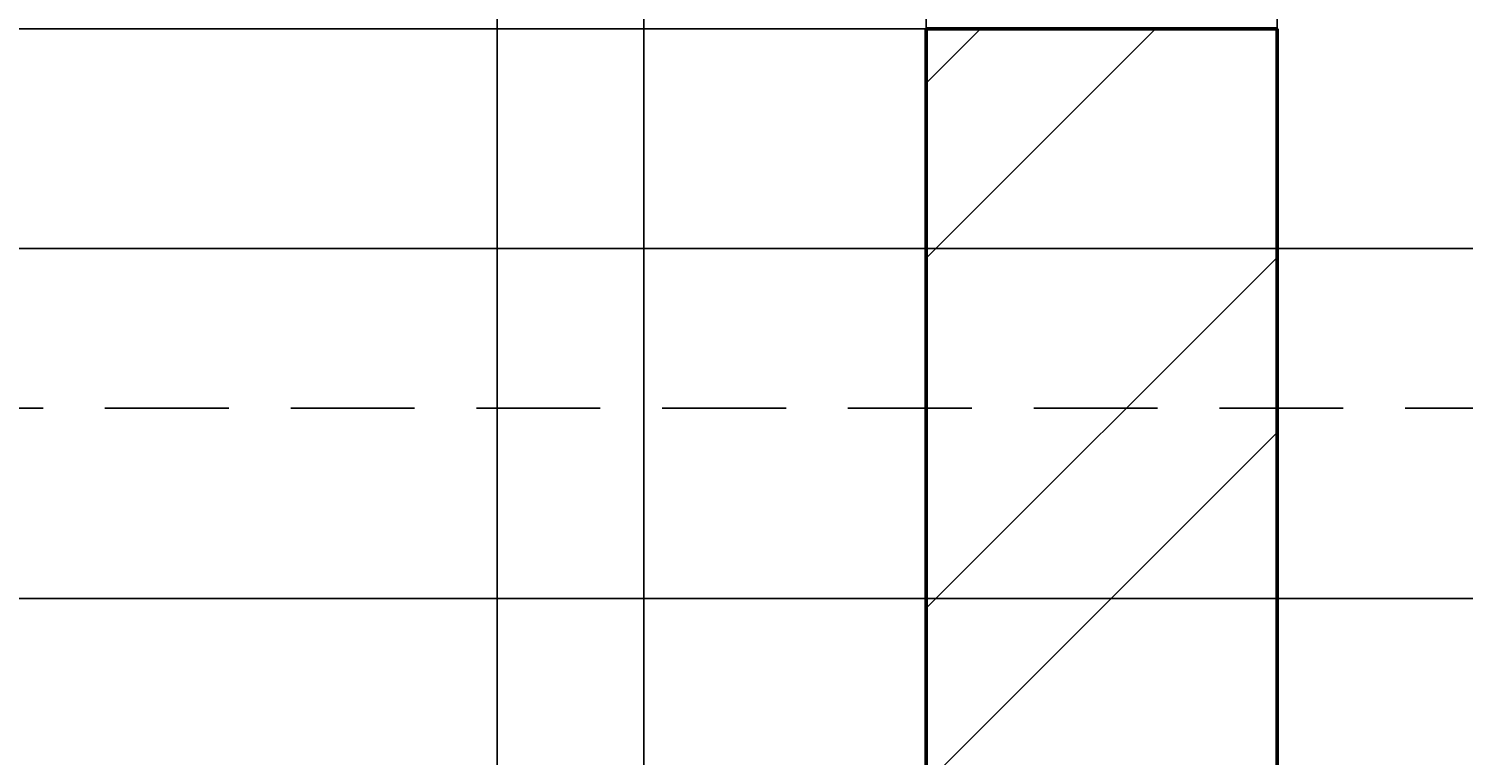
# Model space of a CAD drawing. Units: inches. Extents: x 2812 to 3051, y 1398 to 1659.
# Tile 22 of 65: x 2929 to 2966, y 1453 to 1472. Entities that reach past the tile are written whole.
import ezdxf

# ---------------------------------------------------------------- set-up
doc = ezdxf.new("R2010")
doc.units = ezdxf.units.IN
doc.linetypes.add('HIDDEN2', pattern=[4.7625, 3.175, -1.5875])
for name, color, linetype, lineweight in [('A-ANNO-DIMS', 2, 'Continuous', 18), ('S-CONC', 7, 'Continuous', 50), ('S-CONC-HIDN', 8, 'HIDDEN2', 25), ('S-CONC-PATT', 8, 'Continuous', 18)]:
    doc.layers.add(name, color=color, linetype=linetype, lineweight=lineweight)
doc.styles.get("Standard").update_dxf_attribs({"font": 'arial.ttf'})
doc.dimstyles.get("Standard").update_dxf_attribs({"dimtxt": 0.18, "dimasz": 0.18, "dimexe": 0.18, "dimexo": 0.0625, "dimgap": 0.09, "dimtad": 0, "dimtih": 1, "dimtoh": 1, "dimdec": 4, "dimzin": 0, "dimdsep": 46, "dimtxsty": 'Standard', "dimcen": 0.09, "dimadec": 0, "dimazin": 0, "dimtfac": 1, "dimtdec": 4, "dimtofl": 0, "dimtmove": 0, "dimatfit": 3, "dimfxl": 1, "dimtolj": 1, "dimtzin": 0, "dimarcsym": 0})

# ---------------------------------------------------------------- blocks, each defined once
blk = doc.blocks.new('*D30')
at = {"layer": 'A-ANNO-DIMS', "color": 0, "lineweight": -2, "transparency": 16777216}
for p, q in [((2945.147, 1598.692), (2945.147, 1397.505)), ((2952.385, 1559.757), (2952.385, 1397.505)), ((2945.327, 1397.685), (2948.373, 1397.685)), ((2952.205, 1397.685), (2949.159, 1397.685))]:
    blk.add_line(p, q, dxfattribs=at)
at = {"layer": 'A-ANNO-DIMS', "color": 0, "transparency": 16777216}
for points in [[(2945.327, 1397.715), (2945.327, 1397.655), (2945.147, 1397.685)], [(2952.205, 1397.715), (2952.205, 1397.655), (2952.385, 1397.685)]]:
    blk.add_solid(points, dxfattribs=at)
at = {"layer": 'Defpoints', "color": 0, "transparency": 16777216}
for p in [(2945.147, 1598.754), (2952.385, 1559.82), (2952.385, 1397.685)]:
    blk.add_point(p, dxfattribs=at)
at = {"layer": 'A-ANNO-DIMS', "color": 0, "transparency": 16777216, "insert": (2948.766, 1397.685), "char_height": 0.18, "attachment_point": 5}
blk.add_mtext('\\A1;7.238', dxfattribs=at)
blk = doc.blocks.new('*D31')
at = {"layer": 'A-ANNO-DIMS', "color": 0, "lineweight": -2, "transparency": 16777216}
for p, q in [((2972.272, 1594.192), (2972.272, 1397.505)), ((2961.385, 1559.757), (2961.385, 1397.505)), ((2961.565, 1397.685), (2966.373, 1397.685)), ((2972.092, 1397.685), (2967.283, 1397.685))]:
    blk.add_line(p, q, dxfattribs=at)
at = {"layer": 'A-ANNO-DIMS', "color": 0, "transparency": 16777216}
for points in [[(2961.565, 1397.715), (2961.565, 1397.655), (2961.385, 1397.685)], [(2972.092, 1397.715), (2972.092, 1397.655), (2972.272, 1397.685)]]:
    blk.add_solid(points, dxfattribs=at)
at = {"layer": 'Defpoints', "color": 0, "transparency": 16777216}
for p in [(2972.272, 1594.254), (2961.385, 1559.82), (2972.272, 1397.685)]:
    blk.add_point(p, dxfattribs=at)
at = {"layer": 'A-ANNO-DIMS', "color": 0, "transparency": 16777216, "insert": (2966.828, 1397.685), "char_height": 0.18, "attachment_point": 5}
blk.add_mtext('\\A1;10.887', dxfattribs=at)
blk = doc.blocks.new('*D45')
at = {"layer": 'A-ANNO-DIMS', "color": 0, "lineweight": -2, "transparency": 16777216}
for p, q in [((2896.385, 1487.973), (2896.385, 1397.505)), ((2941.385, 1487.973), (2941.385, 1397.505)), ((2896.565, 1397.685), (2918.662, 1397.685)), ((2941.205, 1397.685), (2919.108, 1397.685))]:
    blk.add_line(p, q, dxfattribs=at)
at = {"layer": 'A-ANNO-DIMS', "color": 0, "transparency": 16777216}
for points in [[(2896.565, 1397.715), (2896.565, 1397.655), (2896.385, 1397.685)], [(2941.205, 1397.715), (2941.205, 1397.655), (2941.385, 1397.685)]]:
    blk.add_solid(points, dxfattribs=at)
at = {"layer": 'Defpoints', "color": 0, "transparency": 16777216}
for p in [(2896.385, 1488.035), (2941.385, 1488.035), (2941.385, 1397.685)]:
    blk.add_point(p, dxfattribs=at)
at = {"layer": 'A-ANNO-DIMS', "color": 0, "transparency": 16777216, "insert": (2918.885, 1397.685), "char_height": 0.18, "attachment_point": 5}
blk.add_mtext('\\A1;45', dxfattribs=at)
blk = doc.blocks.new('*D46')
at = {"layer": 'A-ANNO-DIMS', "color": 0, "lineweight": -2, "transparency": 16777216}
for p, q in [((2941.385, 1487.973), (2941.385, 1397.505)), ((2970.385, 1487.973), (2970.385, 1397.505)), ((2941.565, 1397.685), (2955.664, 1397.685)), ((2970.205, 1397.685), (2956.106, 1397.685))]:
    blk.add_line(p, q, dxfattribs=at)
at = {"layer": 'A-ANNO-DIMS', "color": 0, "transparency": 16777216}
for points in [[(2941.565, 1397.715), (2941.565, 1397.655), (2941.385, 1397.685)], [(2970.205, 1397.715), (2970.205, 1397.655), (2970.385, 1397.685)]]:
    blk.add_solid(points, dxfattribs=at)
at = {"layer": 'Defpoints', "color": 0, "transparency": 16777216}
for p in [(2941.385, 1488.035), (2970.385, 1488.035), (2970.385, 1397.685)]:
    blk.add_point(p, dxfattribs=at)
at = {"layer": 'A-ANNO-DIMS', "color": 0, "transparency": 16777216, "insert": (2955.885, 1397.685), "char_height": 0.18, "attachment_point": 5}
blk.add_mtext('\\A1;29', dxfattribs=at)
blk = doc.blocks.new('*D67')
at = {"layer": 'A-ANNO-DIMS', "color": 0, "lineweight": -2, "transparency": 16777216}
for p, q in [((2906.065, 1457.426), (3051.178, 1457.426)), ((3050.998, 1457.246), (3050.998, 1452.608)), ((3050.998, 1447.606), (3050.998, 1452.245)), ((2914.018, 1447.426), (3051.178, 1447.426))]:
    blk.add_line(p, q, dxfattribs=at)
at = {"layer": 'A-ANNO-DIMS', "color": 0, "transparency": 16777216}
for points in [[(3050.968, 1457.246), (3051.028, 1457.246), (3050.998, 1457.426)], [(3050.968, 1447.606), (3051.028, 1447.606), (3050.998, 1447.426)]]:
    blk.add_solid(points, dxfattribs=at)
at = {"layer": 'Defpoints', "color": 0, "transparency": 16777216}
for p in [(2906.002, 1457.426), (3050.998, 1457.426), (2913.955, 1447.426)]:
    blk.add_point(p, dxfattribs=at)
at = {"layer": 'A-ANNO-DIMS', "color": 0, "transparency": 16777216, "insert": (3050.998, 1452.426), "char_height": 0.18, "attachment_point": 5}
blk.add_mtext('\\A1;10', dxfattribs=at)
blk = doc.blocks.new('*D68')
at = {"layer": 'A-ANNO-DIMS', "color": 0, "lineweight": -2, "transparency": 16777216}
for p, q in [((2898.12, 1466.402), (3051.178, 1466.402)), ((3050.998, 1466.222), (3050.998, 1462.096)), ((3050.998, 1457.606), (3050.998, 1461.733)), ((2906.065, 1457.426), (3051.178, 1457.426))]:
    blk.add_line(p, q, dxfattribs=at)
at = {"layer": 'A-ANNO-DIMS', "color": 0, "transparency": 16777216}
for points in [[(3050.968, 1466.222), (3051.028, 1466.222), (3050.998, 1466.402)], [(3050.968, 1457.606), (3051.028, 1457.606), (3050.998, 1457.426)]]:
    blk.add_solid(points, dxfattribs=at)
at = {"layer": 'Defpoints', "color": 0, "transparency": 16777216}
for p in [(2898.058, 1466.402), (3050.998, 1466.402), (2906.002, 1457.426)]:
    blk.add_point(p, dxfattribs=at)
at = {"layer": 'A-ANNO-DIMS', "color": 0, "transparency": 16777216, "insert": (3050.998, 1461.914), "char_height": 0.18, "attachment_point": 5}
blk.add_mtext('\\A1;8.976', dxfattribs=at)
blk = doc.blocks.new('*D69')
at = {"layer": 'A-ANNO-DIMS', "color": 0, "lineweight": -2, "transparency": 16777216}
for p, q in [((2961.385, 1472.098), (2961.385, 1659.35)), ((2968.956, 1467.81), (2968.956, 1659.35)), ((2961.565, 1659.17), (2964.795, 1659.17)), ((2968.776, 1659.17), (2965.546, 1659.17))]:
    blk.add_line(p, q, dxfattribs=at)
at = {"layer": 'A-ANNO-DIMS', "color": 0, "transparency": 16777216}
for points in [[(2961.565, 1659.2), (2961.565, 1659.14), (2961.385, 1659.17)], [(2968.776, 1659.2), (2968.776, 1659.14), (2968.956, 1659.17)]]:
    blk.add_solid(points, dxfattribs=at)
at = {"layer": 'Defpoints', "color": 0, "transparency": 16777216}
for p in [(2968.956, 1659.17), (2961.385, 1472.035), (2968.956, 1467.747)]:
    blk.add_point(p, dxfattribs=at)
at = {"layer": 'A-ANNO-DIMS', "color": 0, "transparency": 16777216, "insert": (2965.17, 1659.17), "char_height": 0.18, "attachment_point": 5}
blk.add_mtext('\\A1;7.571', dxfattribs=at)
blk = doc.blocks.new('*D77')
at = {"layer": 'A-ANNO-DIMS', "color": 0, "lineweight": -2, "transparency": 16777216}
for p, q in [((2961.322, 1472.035), (2811.806, 1472.035)), ((2811.986, 1471.855), (2811.986, 1461.436)), ((2811.986, 1450.654), (2811.986, 1461.073)), ((2963.812, 1450.474), (2811.806, 1450.474))]:
    blk.add_line(p, q, dxfattribs=at)
at = {"layer": 'A-ANNO-DIMS', "color": 0, "transparency": 16777216}
for points in [[(2811.956, 1471.855), (2812.016, 1471.855), (2811.986, 1472.035)], [(2811.956, 1450.654), (2812.016, 1450.654), (2811.986, 1450.474)]]:
    blk.add_solid(points, dxfattribs=at)
at = {"layer": 'Defpoints', "color": 0, "transparency": 16777216}
for p in [(2811.986, 1472.035), (2961.385, 1472.035), (2963.874, 1450.474)]:
    blk.add_point(p, dxfattribs=at)
at = {"layer": 'A-ANNO-DIMS', "color": 0, "transparency": 16777216, "insert": (2811.986, 1461.255), "char_height": 0.18, "attachment_point": 5}
blk.add_mtext('\\A1;21.56', dxfattribs=at)

msp = doc.modelspace()

# ---------------------------------------------------------------- hatches: boundary and pattern name
at = {"layer": 'S-CONC-PATT'}
h = msp.add_hatch(dxfattribs=at)
h.set_pattern_fill('ANSI32', color=256)
h.paths.add_polyline_path([(3027.3849, 1646.82), (2835.3849, 1646.82), (2835.3849, 1603.2296), (2844.3849, 1603.2296), (2844.3849, 1637.82), (3018.3849, 1637.82), (3018.3849, 1602.5441), (3027.3849, 1602.5441)])
h.paths.add_polyline_path([(2844.3849, 1594.2296), (2835.3849, 1594.2296), (2835.3849, 1550.82), (3027.3849, 1550.82), (3027.3849, 1593.5441), (3018.3849, 1593.5441), (3018.3849, 1559.82), (2844.3849, 1559.82)])
h.paths.add_polyline_path([(2844.3849, 1482.0354), (2835.3849, 1482.0354), (2835.3849, 1463.4959), (2844.3849, 1463.4959)])
h.paths.add_polyline_path([(2844.3849, 1461.4959), (2835.3849, 1461.4959), (2835.3849, 1416.0354), (2844.3849, 1416.0354)])
h.paths.add_polyline_path([(3027.3849, 1482.0354), (3018.3849, 1482.0354), (3018.3849, 1463.2854), (3027.3849, 1463.2854)])
h.paths.add_polyline_path([(3027.3849, 1461.2854), (3018.3849, 1461.2854), (3018.3849, 1416.0354), (3027.3849, 1416.0354)])
h.paths.add_polyline_path([(2961.3849, 1448.4738), (2952.3849, 1448.4738), (2952.3849, 1416.0354), (2961.3849, 1416.0354)])
h.paths.add_polyline_path([(2961.3849, 1462.3026), (2952.3849, 1462.3026), (2952.3849, 1450.4738), (2961.3849, 1450.4738)])
h.paths.add_polyline_path([(2961.3849, 1472.0354), (2952.3849, 1472.0354), (2952.3849, 1462.3026), (2961.3849, 1462.3026)])

# ---------------------------------------------------------------- linework, layer by layer
at = {"layer": 'S-CONC'}
for p, q in [((2952.3849, 1472.0354), (2952.3849, 1416.0354)), ((2952.3849, 1472.0354), (2961.3849, 1472.0354)), ((2961.3849, 1472.0354), (2961.3849, 1450.4738))]:
    msp.add_line(p, q, dxfattribs=at)
at = {"layer": 'S-CONC-HIDN'}
msp.add_line((3029.7562, 1462.3026), (2835.3849, 1462.3026), dxfattribs=at)

# ---------------------------------------------------------------- dimensions: what is measured, and where the dimension line sits
at = {"layer": 'A-ANNO-DIMS'}
for base, p1, p2, override, picture, middle in [((2968.9558, 1659.17), (2961.3849, 1472.0354), (2968.9558, 1467.7474), {"dimdec": 3, "dimlfac": 1, "dimrnd": 0, "dimzin": 0, "dimdsep": 46, "dimlunit": 2}, '*D69', (2965.1704, 1659.17)), ((2952.3849, 1397.6854), (2945.1467, 1598.7541), (2952.3849, 1559.82), {"dimdec": 3, "dimlfac": 1, "dimrnd": 0, "dimzin": 0, "dimdsep": 46, "dimlunit": 2}, '*D30', (2948.7658, 1397.6854)), ((2972.2716, 1397.6854), (2961.3849, 1559.82), (2972.2716, 1594.2541), {"dimdec": 3, "dimlfac": 1, "dimrnd": 0, "dimzin": 0, "dimdsep": 46, "dimlunit": 2}, '*D31', (2966.8282, 1397.6854)), ((2941.3849, 1397.6854), (2896.3849, 1488.0354), (2941.3849, 1488.0354), {"dimdec": 0, "dimlfac": 1, "dimrnd": 0, "dimzin": 0, "dimdsep": 46, "dimlunit": 2}, '*D45', (2918.8849, 1397.6854)), ((2970.3849, 1397.6854), (2941.3849, 1488.0354), (2970.3849, 1488.0354), {"dimdec": 0, "dimlfac": 1, "dimrnd": 0, "dimzin": 0, "dimdsep": 46, "dimlunit": 2}, '*D46', (2955.8849, 1397.6854))]:
    dim = msp.add_linear_dim(base=base, p1=p1, p2=p2, dimstyle='Standard', override=override, dxfattribs=at)
    dim.commit()
    dim.dimension.update_dxf_attribs({"geometry": picture, "text_midpoint": middle})
for base, p1, p2, override, picture, middle in [((2811.9855, 1472.0354), (2963.8741, 1450.4738), (2961.3849, 1472.0354), {"dimdec": 2, "dimlfac": 1, "dimrnd": 0, "dimzin": 0, "dimdsep": 46, "dimlunit": 2}, '*D77', (2811.9855, 1461.2546)), ((3050.998, 1466.4024), (2906.0021, 1457.4265), (2898.0577, 1466.4024), {"dimdec": 3, "dimlfac": 1, "dimrnd": 0, "dimzin": 0, "dimdsep": 46, "dimlunit": 2}, '*D68', (3050.998, 1461.9144)), ((3050.998, 1457.4265), (2913.9551, 1447.4265), (2906.0021, 1457.4265), {"dimdec": 0, "dimlfac": 1, "dimrnd": 0, "dimzin": 0, "dimdsep": 46, "dimlunit": 2}, '*D67', (3050.998, 1452.4265))]:
    dim = msp.add_linear_dim(base=base, p1=p1, p2=p2, angle=90, dimstyle='Standard', override=override, dxfattribs=at)
    dim.commit()
    dim.dimension.update_dxf_attribs({"geometry": picture, "text_midpoint": middle})

doc.saveas('drawing.dxf')
